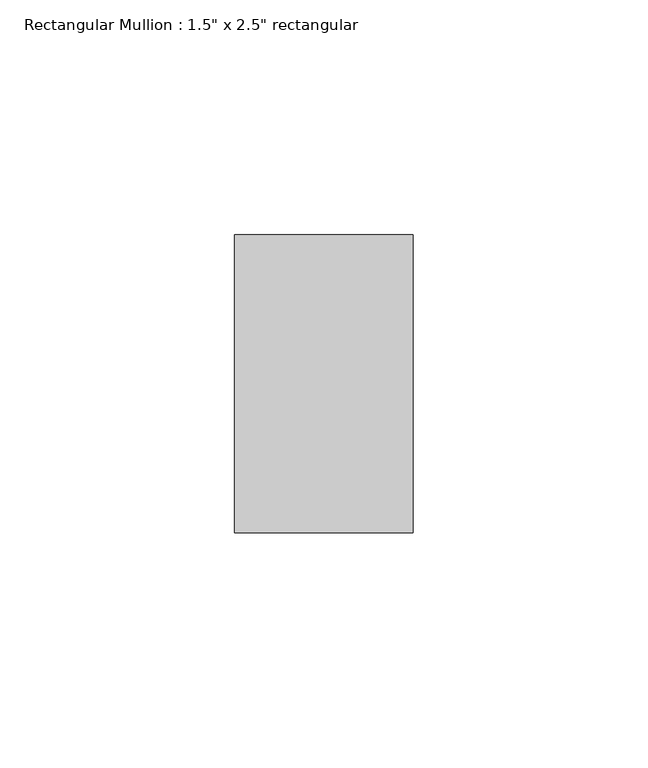
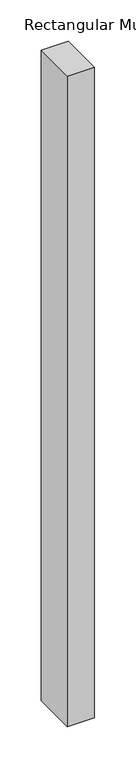
"""IFC4 building model written with IfcOpenShell, lengths in millimetres: member geometry."""

from ifc_helpers import new_model, si_unit, frame, origin, place, context, project, spatial, polyline, outline, extrude, source, transform, mapped, element, save


def member_1ede677d(model_context):
    return source(origin(), model_context, "Body", "SweptSolid", [
        extrude(outline(polyline([(19.05, 31.75), (19.05, -31.75), (-19.05, -31.75), (-19.05, 31.75), (19.05, 31.75)])), frame((0.0, 0.0, -965.2), z_axis=(0.0, 0.0, 1.0), x_axis=(1.0, 0.0, 0.0)), (0.0, 0.0, 1.0), 965.2),
    ])


if __name__ == "__main__":
    model = new_model("IFC4")
    model_context = context("Model", 3, world=origin())
    ifc_project = project(units=[si_unit("LENGTHUNIT", "METRE", prefix="MILLI")], contexts=[model_context])
    site = spatial("IfcSite", under=ifc_project)
    building = spatial("IfcBuilding", under=site)
    placement = place(None, origin())
    member_shape = member_1ede677d(model_context)
    element("IfcMember", 1, ObjectType="Rectangular Mullion : 1.5\" x 2.5\" rectangular", at=placement, inside=building, context=model_context, shape_type="MappedRepresentation", body=[
        mapped(member_shape, transform((0.0, 0.0, 0.0), x_axis=(1.0, 0.0, 0.0), y_axis=(0.0, 1.0, 0.0), z_axis=(0.0, 0.0, 1.0))),
    ])
    save(model, "model.ifc")

# Revit data of these elements
# Type "Rectangular Mullion : 1.5\" x 2.5\" rectangular"
#   built-in parameter 1007304 = 0.208333 (stored number, unit not read)
#   built-in parameter 1007301 = 0.0625 (stored number, unit not read)
#   built-in parameter 1007300 = 0.0625 (stored number, unit not read)
# Element 1 (IfcMember, "Rectangular Mullion : 1.5\" x 2.5\" rectangular")
#   Materials on its faces: "Aluminum"
# Materials
#   "Aluminum": class "Metal", colour RGB 247 247 247, transparency 0, Description = "Aluminum 6061", Cost = 0
